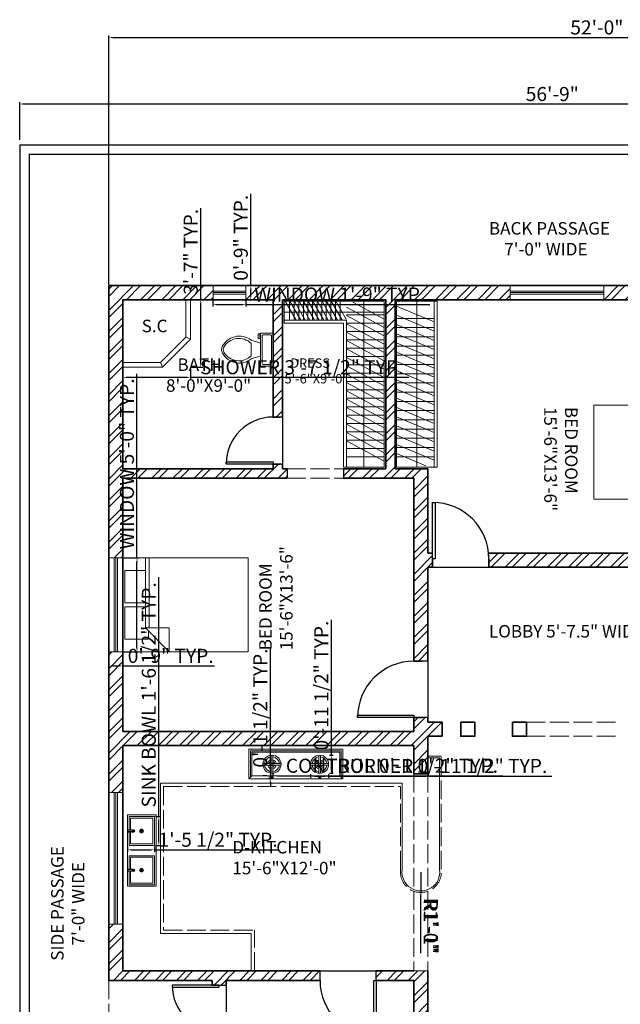
# Model space of a CAD drawing. Units: inches. Extents: x 839 to 1638, y 2998 to 4342.
# Tile 3 of 4: x 839 to 1223, y 3713 to 4342. Entities that reach past the tile are written whole.
import ezdxf

# ---------------------------------------------------------------- set-up
doc = ezdxf.new("R2010")
doc.units = ezdxf.units.IN
doc.linetypes.add('ACAD_ISO02W100', pattern=[15, 12, -3])
for name, color, linetype, lineweight in [('A-ANNO-DIMS', 2, 'Continuous', 18), ('A-AREA-IDEN', 7, 'Continuous', 18), ('A-COLS', 7, 'Continuous', 35), ('A-DOOR', 4, 'Continuous', 25), ('A-DOOR-JAMB', 7, 'Continuous', 25), ('A-EQPM', 8, 'Continuous', 18), ('A-FLOR-CASE', 9, 'Continuous', 20), ('A-FLOR-CASE-HIDN', 9, 'ACAD_ISO02W100', 13), ('A-FLOR-CASE-PATT', 252, 'Continuous', 13), ('A-FLOR-FIXT', 9, 'Continuous', 18), ('A-FLOR-OVHD', 8, 'ACAD_ISO02W100', 18), ('A-FURN', 8, 'Continuous', 18), ('A-WALL', 7, 'Continuous', 35), ('A-WALL-OVHD', 8, 'ACAD_ISO02W100', 18), ('A-WALL-PATT', 252, 'Continuous', 13), ('C-PROP', 7, 'Continuous', 30)]:
    doc.layers.add(name, color=color, linetype=linetype, lineweight=lineweight)
doc.layers.add('A-GLAZ', color=244, linetype='Continuous', lineweight=20, true_color=0x991b1e)
doc.styles.get("Standard").update_dxf_attribs({"font": 'arial.ttf'})
doc.dimstyles.new('ISO-25', dxfattribs={"dimtxt": 9, "dimasz": 2.5, "dimexe": 1.25, "dimexo": 0.625, "dimtad": 1, "dimlunit": 3, "dimtxsty": 'Standard', "dimcen": 2.5, "dimadec": 0, "dimazin": 0, "dimtfac": 1, "dimtmove": 0, "dimatfit": 3, "dimfxl": 1, "dimarcsym": 0})

# ---------------------------------------------------------------- blocks, each defined once
blk = doc.blocks.new('*U2')
for p, q in [((0, 0), (0, -6)), ((40, 0), (40, -6))]:
    blk.add_line(p, q)
blk.add_lwpolyline([(0, 0), (0, 40), (1.75, 40), (1.75, 0)], close=True)
blk.add_arc((0, 0), 40, 0, 90)
blk = doc.blocks.new('*U5')
for p, q in [((0, 0), (0, -6)), ((40, 0), (40, -6))]:
    blk.add_line(p, q)
blk.add_lwpolyline([(0, 0), (0, 40), (1.75, 40), (1.75, 0)], close=True)
blk.add_arc((0, 0), 40, 0, 90)
blk = doc.blocks.new('*U7')
for p, q in [((-40, 0), (-40, 6)), ((0, 0), (0, 6))]:
    blk.add_line(p, q)
blk.add_lwpolyline([(0, 0), (0, -40), (-1.75, -40), (-1.75, 0)], close=True)
blk.add_arc((0, 0), 40, 180, 270)
blk = doc.blocks.new('*U9')
for p, q in [((-40, 0), (-40, 6)), ((0, 0), (0, 6))]:
    blk.add_line(p, q)
blk.add_lwpolyline([(0, 0), (0, -40), (-1.75, -40), (-1.75, 0)], close=True)
blk.add_arc((0, 0), 40, 180, 270)
blk = doc.blocks.new('*U10')
for p, q in [((0, 0), (0, 6)), ((40, 0), (40, 6))]:
    blk.add_line(p, q)
blk.add_lwpolyline([(0, 0), (0, -40), (1.75, -40), (1.75, 0)], close=True)
blk.add_arc((0, 0), 40, 270, 360)
blk = doc.blocks.new('Bed - Queen')
for p, q in [((0, -80.00003), (0, 0)), ((0, 0), (59.99999, 0)), ((59.99999, 0), (59.99999, -80.00003)), ((7.99999, -1.2), (28.79998, -1.2)), ((7.99999, -14.4), (7.99999, -1.2)), ((28.79998, -1.2), (28.79998, -14.4)), ((31.19999, -1.2), (51.99999, -1.2)), ((31.19999, -14.4), (31.19999, -1.2)), ((51.99999, -1.2), (51.99999, -16.4)), ((0, -14.4), (44.8, -14.4)), ((44.8, -16.8), (0, -16.8)), ((59.99999, -29.6), (44.8, -14.4)), ((44.8, -14.4), (44.8, -29.6)), ((51.99999, -16.4), (46.79936, -16.4)), ((44.8, -29.6), (59.99999, -29.6)), ((59.99999, -80.00003), (0, -80.00003))]:
    blk.add_line(p, q)
blk = doc.blocks.new('*U15')
for p, q in [((9.5, -6), (9.5, -2)), ((-10, -8.5), (-8, -8.5)), ((-10, -9.5), (-10, -8.5)), ((-7, -9.5), (-10, -9.5)), ((-8, -8.5), (-8, -8)), ((-7, -8), (-7, -9.5)), ((-4, -8), (-6, -14)), ((4, -8), (6, -14)), ((4, -14), (-4, -14))]:
    blk.add_line(p, q)
blk.add_lwpolyline([(10.5, -8), (10.5, 0), (-10.5, 0), (-10.5, -8)], close=True)
for points in [[(-9.5, -2), (-9.5, -6)], [(8.5, -1), (-8.5, -1)], [(-8.5, -7), (8.5, -7)]]:
    blk.add_lwpolyline(points)
for centre, radius, start, end in [((-8.62, -1.88), 0.884, 81.8699, 188.1301), ((-8.62, -6.12), 0.884, 171.8699, 278.1301), ((8.62, -1.88), 0.884, 351.8699, 98.1301), ((8.62, -6.12), 0.884, 261.8699, 8.1301), ((3.52, -21.58), 12.17, 141.46911, 247.97143), ((4.2, -21.82), 11.33, 136.36773, 238.94682), ((-3.52, -21.58), 12.17, 292.02843, 38.53071), ((-4.2, -21.82), 11.33, 301.05301, 43.63209), ((0, -27.88), 4, 245.73182, 294.26817), ((0, -29), 4, 254.86053, 285.13947)]:
    blk.add_arc(centre, radius, start, end)
blk = doc.blocks.new('*D20')
at = {"layer": 'A-ANNO-DIMS', "color": 0, "lineweight": -2, "transparency": 16777216}
for p, q in [((839.17, 4265.09), (839.17, 4289.16)), ((841.67, 4287.91), (1517.67, 4287.91)), ((1520.17, 4265.46), (1520.17, 4289.16))]:
    blk.add_line(p, q, dxfattribs=at)
at = {"layer": 'A-ANNO-DIMS', "color": 0, "transparency": 16777216}
for points in [[(841.67, 4288.33), (841.67, 4287.5), (839.17, 4287.91)], [(1517.67, 4288.33), (1517.67, 4287.5), (1520.17, 4287.91)]]:
    blk.add_solid(points, dxfattribs=at)
at = {"layer": 'Defpoints', "color": 0, "transparency": 16777216}
for p in [(1520.17, 4287.91), (839.17, 4264.46), (1520.17, 4264.84)]:
    blk.add_point(p, dxfattribs=at)
at = {"layer": 'A-ANNO-DIMS', "color": 0, "transparency": 16777216, "insert": (1179.67, 4293.13), "char_height": 9, "attachment_point": 5}
blk.add_mtext('56\'-9"', dxfattribs=at)
blk = doc.blocks.new('WIN-60x9')
for p, q in [((3.5, 60), (3.5, 0)), ((4.5, 60), (4.5, 0)), ((5.5, 60), (5.5, 0))]:
    blk.add_line(p, q)
blk.add_lwpolyline([(9, 60), (9, 0), (0, 0), (0, 60)], close=True)
blk = doc.blocks.new('WIN-21x9')
for p, q in [((0, 5.5), (21, 5.5)), ((0, 4.5), (21, 4.5)), ((0, 3.5), (21, 3.5))]:
    blk.add_line(p, q)
blk.add_lwpolyline([(0, 9), (21, 9), (21, 0), (0, 0)], close=True)
blk = doc.blocks.new('POST-9x9')
blk.add_lwpolyline([(0, 9), (9, 9), (9, 0), (0, 0)], close=True)
blk = doc.blocks.new('SHOWER-CORNER')
for p, q in [((40.25, 43.12), (40.25, 19.12)), ((43.25, 43.12), (43.25, 17.87)), ((24, 3), (40.25, 19.12)), ((40.25, 19.12), (43.25, 17.87)), ((25.23, 0), (43.25, 17.87)), ((0, 3), (24, 3)), ((0, 0), (25.23, 0)), ((24, 3), (25.23, 0))]:
    blk.add_line(p, q)
blk = doc.blocks.new('SINK-BOWL-WITH-TAP')
for p, q in [((0, 9.97), (3.7, 9.97)), ((0, 9.67), (3.31, 9.67)), ((0, 8.87), (3.31, 8.87)), ((0, 8.57), (3.7, 8.57)), ((7.73, 9.27), (10.16, 9.27)), ((9.8, 8.4), (8.09, 10.14)), ((8.15, 8.35), (9.75, 10.19)), ((8.95, 10.49), (8.95, 8.05))]:
    blk.add_line(p, q)
for points in [[(1, 9.97), (1, 18.54), (17.27, 18.54), (17.27, 0), (1, 0), (1, 8.57)], [(2, 9.97), (2, 17.54), (16.27, 17.54), (16.27, 1), (2, 1), (2, 8.57)]]:
    blk.add_lwpolyline(points)
for centre, radius in [((3.93, 9.27), 0.739), ((3.93, 9.27), 0.439), ((8.95, 9.27), 1.22), ((8.95, 9.27), 0.619)]:
    blk.add_circle(centre, radius)
blk = doc.blocks.new('COOKTOP-BURNER')
for p, q in [((5.27, 11.54), (5.27, 0)), ((6.27, 11.54), (6.27, 0)), ((0, 6.27), (11.54, 6.27)), ((0, 5.27), (11.54, 5.27))]:
    blk.add_line(p, q)
blk.add_circle((5.77, 5.77), 5.77)
for radius, start, end in [(4.77, 96.01576, 173.98424), (2.77, 100.39579, 169.60421), (1.77, 106.40006, 163.59994), (4.77, 6.01576, 83.98424), (2.77, 10.39579, 79.60421), (1.77, 16.40006, 73.59994), (4.77, 186.01576, 263.98424), (2.77, 190.39579, 259.60421), (1.77, 196.40006, 253.59994), (1.77, 286.40006, 343.59994), (2.77, 280.39579, 349.60421), (4.77, 276.01576, 353.98424)]:
    blk.add_arc((5.77, 5.77), radius, start, end)
blk = doc.blocks.new('COOKTOP-CONTROL')
for p, q in [((0.03, 0.97), (1.52, 0.97)), ((0.03, 0.57), (1.52, 0.57))]:
    blk.add_line(p, q)
blk.add_circle((0.77, 0.77), 0.771)
for start, end in [(25.1412, 154.8588), (205.1412, 334.8588)]:
    blk.add_arc((0.77, 0.77), 0.471, start, end)
blk = doc.blocks.new('*D32')
at = {"layer": 'A-ANNO-DIMS', "color": 0, "lineweight": -2, "transparency": 16777216}
for p, q in [((962.76, 4162.21), (962.76, 4158.44)), ((965.26, 4159.69), (981.26, 4159.69)), ((983.76, 4162.21), (983.76, 4158.44)), ((983.76, 4159.69), (1101.4, 4159.69))]:
    blk.add_line(p, q, dxfattribs=at)
at = {"layer": 'A-ANNO-DIMS', "color": 0, "transparency": 16777216}
for points in [[(965.26, 4160.1), (965.26, 4159.27), (962.76, 4159.69)], [(981.26, 4160.1), (981.26, 4159.27), (983.76, 4159.69)]]:
    blk.add_solid(points, dxfattribs=at)
at = {"layer": 'Defpoints', "color": 0, "transparency": 16777216}
for p in [(962.76, 4162.84), (983.76, 4162.84), (983.76, 4159.69)]:
    blk.add_point(p, dxfattribs=at)
at = {"layer": 'A-ANNO-DIMS', "color": 0, "transparency": 16777216, "insert": (1043.83, 4164.97), "char_height": 9, "attachment_point": 5}
blk.add_mtext('WINDOW 1\'-9" TYP.', dxfattribs=at)
blk = doc.blocks.new('*D33')
at = {"layer": 'A-ANNO-DIMS', "color": 0, "lineweight": -2, "transparency": 16777216}
for p, q in [((986.91, 4171.84), (986.91, 4230.45)), ((984.39, 4171.84), (988.16, 4171.84)), ((986.91, 4165.34), (986.91, 4169.34)), ((984.39, 4162.84), (988.16, 4162.84))]:
    blk.add_line(p, q, dxfattribs=at)
at = {"layer": 'A-ANNO-DIMS', "color": 0, "transparency": 16777216}
for points in [[(986.5, 4169.34), (987.33, 4169.34), (986.91, 4171.84)], [(986.5, 4165.34), (987.33, 4165.34), (986.91, 4162.84)]]:
    blk.add_solid(points, dxfattribs=at)
at = {"layer": 'Defpoints', "color": 0, "transparency": 16777216}
for p in [(983.76, 4171.84), (986.91, 4171.84), (983.76, 4162.84)]:
    blk.add_point(p, dxfattribs=at)
at = {"layer": 'A-ANNO-DIMS', "color": 0, "transparency": 16777216, "insert": (981.69, 4202.39), "char_height": 9, "attachment_point": 5, "rotation": 90}
blk.add_mtext('0\'-9" TYP.', dxfattribs=at)
blk = doc.blocks.new('*D36')
at = {"layer": 'A-ANNO-DIMS', "color": 0, "lineweight": -2, "transparency": 16777216}
for p, q in [((914.17, 3997.84), (914.17, 4115.47)), ((905.79, 3997.84), (915.42, 3997.84)), ((914.17, 3940.34), (914.17, 3995.34)), ((905.79, 3937.84), (915.42, 3937.84))]:
    blk.add_line(p, q, dxfattribs=at)
at = {"layer": 'A-ANNO-DIMS', "color": 0, "transparency": 16777216}
for points in [[(913.75, 3995.34), (914.59, 3995.34), (914.17, 3997.84)], [(913.75, 3940.34), (914.59, 3940.34), (914.17, 3937.84)]]:
    blk.add_solid(points, dxfattribs=at)
at = {"layer": 'Defpoints', "color": 0, "transparency": 16777216}
for p in [(905.17, 3997.84), (914.17, 3997.84), (905.17, 3937.84)]:
    blk.add_point(p, dxfattribs=at)
at = {"layer": 'A-ANNO-DIMS', "color": 0, "transparency": 16777216, "insert": (908.89, 4057.9), "char_height": 9, "attachment_point": 5, "rotation": 90}
blk.add_mtext('WINDOW 5\'-0" TYP.', dxfattribs=at)
blk = doc.blocks.new('*D37')
at = {"layer": 'A-ANNO-DIMS', "color": 0, "lineweight": -2, "transparency": 16777216}
for p, q in [((896.17, 3937.21), (896.17, 3927.59)), ((905.17, 3937.21), (905.17, 3927.59)), ((898.67, 3928.84), (902.67, 3928.84)), ((905.17, 3928.84), (963.78, 3928.84))]:
    blk.add_line(p, q, dxfattribs=at)
at = {"layer": 'A-ANNO-DIMS', "color": 0, "transparency": 16777216}
for points in [[(898.67, 3929.25), (898.67, 3928.42), (896.17, 3928.84)], [(902.67, 3929.25), (902.67, 3928.42), (905.17, 3928.84)]]:
    blk.add_solid(points, dxfattribs=at)
at = {"layer": 'Defpoints', "color": 0, "transparency": 16777216}
for p in [(896.17, 3937.84), (905.17, 3937.84), (905.17, 3928.84)]:
    blk.add_point(p, dxfattribs=at)
at = {"layer": 'A-ANNO-DIMS', "color": 0, "transparency": 16777216, "insert": (935.72, 3934.06), "char_height": 9, "attachment_point": 5}
blk.add_mtext('0\'-9" TYP.', dxfattribs=at)
blk = doc.blocks.new('*D38')
at = {"layer": 'A-ANNO-DIMS', "color": 0, "lineweight": -2, "transparency": 16777216}
for p, q in [((905.17, 4119.09), (905.17, 4111.98)), ((948.42, 4119.09), (948.42, 4111.98)), ((907.67, 4113.23), (945.92, 4113.23)), ((948.42, 4113.23), (1088.03, 4113.23))]:
    blk.add_line(p, q, dxfattribs=at)
at = {"layer": 'A-ANNO-DIMS', "color": 0, "transparency": 16777216}
for points in [[(907.67, 4113.65), (907.67, 4112.81), (905.17, 4113.23)], [(945.92, 4113.65), (945.92, 4112.81), (948.42, 4113.23)]]:
    blk.add_solid(points, dxfattribs=at)
at = {"layer": 'Defpoints', "color": 0, "transparency": 16777216}
for p in [(905.17, 4119.72), (948.42, 4119.72), (948.42, 4113.23)]:
    blk.add_point(p, dxfattribs=at)
at = {"layer": 'A-ANNO-DIMS', "color": 0, "transparency": 16777216, "insert": (1019.48, 4118.51), "char_height": 9, "attachment_point": 5}
blk.add_mtext('SHOWER 3\'-7 1/2" TYP.', dxfattribs=at)
blk = doc.blocks.new('*D39')
at = {"layer": 'A-ANNO-DIMS', "color": 0, "lineweight": -2, "transparency": 16777216}
for p, q in [((954.91, 4162.84), (954.91, 4221.44)), ((949.05, 4162.84), (956.16, 4162.84)), ((954.91, 4122.22), (954.91, 4160.34)), ((949.05, 4119.72), (956.16, 4119.72))]:
    blk.add_line(p, q, dxfattribs=at)
at = {"layer": 'A-ANNO-DIMS', "color": 0, "transparency": 16777216}
for points in [[(954.49, 4160.34), (955.33, 4160.34), (954.91, 4162.84)], [(954.49, 4122.22), (955.33, 4122.22), (954.91, 4119.72)]]:
    blk.add_solid(points, dxfattribs=at)
at = {"layer": 'Defpoints', "color": 0, "transparency": 16777216}
for p in [(948.42, 4162.84), (954.91, 4162.84), (948.42, 4119.72)]:
    blk.add_point(p, dxfattribs=at)
at = {"layer": 'A-ANNO-DIMS', "color": 0, "transparency": 16777216, "insert": (949.69, 4193.39), "char_height": 9, "attachment_point": 5, "rotation": 90}
blk.add_mtext('3\'-7" TYP.', dxfattribs=at)
blk = doc.blocks.new('*D40')
at = {"layer": 'A-ANNO-DIMS', "color": 0, "lineweight": -2, "transparency": 16777216}
for p, q in [((928.15, 3832.6), (928.15, 3985.49)), ((926, 3832.6), (929.4, 3832.6)), ((928.15, 3816.56), (928.15, 3830.1)), ((926, 3814.06), (929.4, 3814.06))]:
    blk.add_line(p, q, dxfattribs=at)
at = {"layer": 'A-ANNO-DIMS', "color": 0, "transparency": 16777216}
for points in [[(927.74, 3830.1), (928.57, 3830.1), (928.15, 3832.6)], [(927.74, 3816.56), (928.57, 3816.56), (928.15, 3814.06)]]:
    blk.add_solid(points, dxfattribs=at)
at = {"layer": 'Defpoints', "color": 0, "transparency": 16777216}
for p in [(925.37, 3832.6), (928.15, 3832.6), (925.37, 3814.06)]:
    blk.add_point(p, dxfattribs=at)
at = {"layer": 'A-ANNO-DIMS', "color": 0, "transparency": 16777216, "insert": (922.87, 3910.3), "char_height": 9, "attachment_point": 5, "rotation": 90}
blk.add_mtext('SINK BOWL 1\'-6 1/2" TYP.', dxfattribs=at)
blk = doc.blocks.new('*D41')
at = {"layer": 'A-ANNO-DIMS', "color": 0, "lineweight": -2, "transparency": 16777216}
for p, q in [((908.11, 3813.43), (908.11, 3810.03)), ((925.37, 3813.43), (925.37, 3810.03)), ((910.61, 3811.28), (922.87, 3811.28)), ((925.37, 3811.28), (1004.11, 3811.28))]:
    blk.add_line(p, q, dxfattribs=at)
at = {"layer": 'A-ANNO-DIMS', "color": 0, "transparency": 16777216}
for points in [[(910.61, 3811.69), (910.61, 3810.86), (908.11, 3811.28)], [(922.87, 3811.69), (922.87, 3810.86), (925.37, 3811.28)]]:
    blk.add_solid(points, dxfattribs=at)
at = {"layer": 'Defpoints', "color": 0, "transparency": 16777216}
for p in [(908.11, 3814.06), (925.37, 3814.06), (925.37, 3811.28)]:
    blk.add_point(p, dxfattribs=at)
at = {"layer": 'A-ANNO-DIMS', "color": 0, "transparency": 16777216, "insert": (965.99, 3816.56), "char_height": 9, "attachment_point": 5}
blk.add_mtext('1\'-5 1/2" TYP.', dxfattribs=at)
blk = doc.blocks.new('*D42')
at = {"layer": 'A-ANNO-DIMS', "color": 0, "lineweight": -2, "transparency": 16777216}
for p, q in [((1025.15, 3859.53), (1025.15, 3857.18)), ((1027.65, 3858.43), (1034.19, 3858.43)), ((1036.69, 3859.53), (1036.69, 3857.18)), ((1036.69, 3858.43), (1179.45, 3858.43))]:
    blk.add_line(p, q, dxfattribs=at)
at = {"layer": 'A-ANNO-DIMS', "color": 0, "transparency": 16777216}
for points in [[(1027.65, 3858.84), (1027.65, 3858.01), (1025.15, 3858.43)], [(1034.19, 3858.84), (1034.19, 3858.01), (1036.69, 3858.43)]]:
    blk.add_solid(points, dxfattribs=at)
at = {"layer": 'Defpoints', "color": 0, "transparency": 16777216}
for p in [(1025.15, 3860.16), (1036.69, 3860.16), (1036.69, 3858.43)]:
    blk.add_point(p, dxfattribs=at)
at = {"layer": 'A-ANNO-DIMS', "color": 0, "transparency": 16777216, "insert": (1109.32, 3863.7), "char_height": 9, "attachment_point": 5}
blk.add_mtext('BURNER 0\'-11 1/2" TYP.', dxfattribs=at)
blk = doc.blocks.new('*D43')
at = {"layer": 'A-ANNO-DIMS', "color": 0, "lineweight": -2, "transparency": 16777216}
for p, q in [((1038.42, 3871.7), (1038.42, 3958.27)), ((1037.32, 3871.7), (1039.67, 3871.7)), ((1038.42, 3862.66), (1038.42, 3869.2)), ((1037.32, 3860.16), (1039.67, 3860.16))]:
    blk.add_line(p, q, dxfattribs=at)
at = {"layer": 'A-ANNO-DIMS', "color": 0, "transparency": 16777216}
for points in [[(1038.01, 3869.2), (1038.84, 3869.2), (1038.42, 3871.7)], [(1038.01, 3862.66), (1038.84, 3862.66), (1038.42, 3860.16)]]:
    blk.add_solid(points, dxfattribs=at)
at = {"layer": 'Defpoints', "color": 0, "transparency": 16777216}
for p in [(1036.69, 3871.7), (1038.42, 3871.7), (1036.69, 3860.16)]:
    blk.add_point(p, dxfattribs=at)
at = {"layer": 'A-ANNO-DIMS', "color": 0, "transparency": 16777216, "insert": (1033.14, 3916.24), "char_height": 9, "attachment_point": 5, "rotation": 90}
blk.add_mtext('0\'-11 1/2" TYP.', dxfattribs=at)
blk = doc.blocks.new('*D44')
at = {"layer": 'A-ANNO-DIMS', "color": 0, "lineweight": -2, "transparency": 16777216}
for p, q in [((997.15, 3858.56), (994.65, 3858.56)), ((999.65, 3858.96), (999.65, 3859.81)), ((999.65, 3858.56), (1001.19, 3858.56)), ((1001.19, 3858.96), (1001.19, 3859.81)), ((1003.69, 3858.56), (1148.13, 3858.56))]:
    blk.add_line(p, q, dxfattribs=at)
at = {"layer": 'A-ANNO-DIMS', "color": 0, "transparency": 16777216}
for points in [[(997.15, 3858.98), (997.15, 3858.15), (999.65, 3858.56)], [(1003.69, 3858.98), (1003.69, 3858.15), (1001.19, 3858.56)]]:
    blk.add_solid(points, dxfattribs=at)
at = {"layer": 'Defpoints', "color": 0, "transparency": 16777216}
for p in [(999.65, 3858.33), (1001.19, 3858.56), (1001.19, 3858.33)]:
    blk.add_point(p, dxfattribs=at)
at = {"layer": 'A-ANNO-DIMS', "color": 0, "transparency": 16777216, "insert": (1077.16, 3863.84), "char_height": 9, "attachment_point": 5}
blk.add_mtext('CONTROL 0\'-1 1/2" TYP.', dxfattribs=at)
blk = doc.blocks.new('*D45')
at = {"layer": 'A-ANNO-DIMS', "color": 0, "lineweight": -2, "transparency": 16777216}
for p, q in [((999.42, 3860.83), (999.42, 3940.41)), ((999.02, 3858.33), (998.17, 3858.33)), ((999.42, 3856.79), (999.42, 3858.33)), ((999.02, 3856.79), (998.17, 3856.79)), ((999.42, 3854.29), (999.42, 3851.79))]:
    blk.add_line(p, q, dxfattribs=at)
at = {"layer": 'A-ANNO-DIMS', "color": 0, "transparency": 16777216}
for points in [[(999, 3860.83), (999.83, 3860.83), (999.42, 3858.33)], [(999, 3854.29), (999.83, 3854.29), (999.42, 3856.79)]]:
    blk.add_solid(points, dxfattribs=at)
at = {"layer": 'Defpoints', "color": 0, "transparency": 16777216}
for p in [(999.42, 3858.33), (999.65, 3858.33), (999.65, 3856.79)]:
    blk.add_point(p, dxfattribs=at)
at = {"layer": 'A-ANNO-DIMS', "color": 0, "transparency": 16777216, "insert": (994.14, 3901.87), "char_height": 9, "attachment_point": 5, "rotation": 90}
blk.add_mtext('0\'-1 1/2" TYP.', dxfattribs=at)
blk = doc.blocks.new('*D50')
at = {"layer": 'A-ANNO-DIMS', "color": 0, "lineweight": -2, "transparency": 16777216}
for p, q in [((896.17, 4172.46), (896.17, 4331.69)), ((898.67, 4330.44), (1517.67, 4330.44)), ((1520.17, 4265.46), (1520.17, 4331.69))]:
    blk.add_line(p, q, dxfattribs=at)
at = {"layer": 'A-ANNO-DIMS', "color": 0, "transparency": 16777216}
for points in [[(898.67, 4330.85), (898.67, 4330.02), (896.17, 4330.44)], [(1517.67, 4330.85), (1517.67, 4330.02), (1520.17, 4330.44)]]:
    blk.add_solid(points, dxfattribs=at)
at = {"layer": 'Defpoints', "color": 0, "transparency": 16777216}
for p in [(1520.17, 4330.44), (1520.17, 4264.84), (896.17, 4171.84)]:
    blk.add_point(p, dxfattribs=at)
at = {"layer": 'A-ANNO-DIMS', "color": 0, "transparency": 16777216, "insert": (1208.17, 4335.66), "char_height": 9, "attachment_point": 5}
blk.add_mtext('52\'-0"', dxfattribs=at)
blk = doc.blocks.new('*D52')
at = {"layer": 'A-ANNO-DIMS', "color": 0, "lineweight": -2, "transparency": 16777216}
for p, q in [((1095.67, 3797.09), (1095.67, 3783.99)), ((1095.67, 3745.2), (1095.67, 3781.49))]:
    blk.add_line(p, q, dxfattribs=at)
at = {"layer": 'A-ANNO-DIMS', "color": 0, "transparency": 16777216}
blk.add_solid([(1096.09, 3781.49), (1095.25, 3781.49), (1095.67, 3783.99)], dxfattribs=at)
at = {"layer": 'Defpoints', "color": 0, "transparency": 16777216}
for p in [(1095.67, 3797.09), (1095.67, 3783.99)]:
    blk.add_point(p, dxfattribs=at)
at = {"layer": 'A-ANNO-DIMS', "color": 0, "transparency": 16777216, "insert": (1100.81, 3762.1), "char_height": 9, "attachment_point": 5, "rotation": 270.00202}
blk.add_mtext('R1\'-1"', dxfattribs=at)
blk = doc.blocks.new('*D53')
at = {"layer": 'A-ANNO-DIMS', "color": 0, "lineweight": -2, "transparency": 16777216}
for p, q in [((1095.67, 3797.09), (1095.67, 3784.99)), ((1095.67, 3746.2), (1095.67, 3782.49))]:
    blk.add_line(p, q, dxfattribs=at)
at = {"layer": 'A-ANNO-DIMS', "color": 0, "transparency": 16777216}
blk.add_solid([(1096.09, 3782.49), (1095.25, 3782.49), (1095.67, 3784.99)], dxfattribs=at)
at = {"layer": 'Defpoints', "color": 0, "transparency": 16777216}
for p in [(1095.67, 3797.09), (1095.67, 3784.99)]:
    blk.add_point(p, dxfattribs=at)
at = {"layer": 'A-ANNO-DIMS', "color": 0, "transparency": 16777216, "insert": (1100.89, 3763.1), "char_height": 9, "attachment_point": 5, "rotation": 270.00219}
blk.add_mtext('R1\'-0"', dxfattribs=at)

msp = doc.modelspace()

# ---------------------------------------------------------------- hatches: boundary and pattern name
at = {"layer": 'A-FLOR-CASE-PATT'}
h = msp.add_hatch(dxfattribs=at)
h.set_pattern_fill('ANSI31', color=256, scale=0.8000071, angle=74.98736, style=0)
h.paths.add_polyline_path([(1008.169, 4161.836), (1015.093, 4149.836), (1047.352, 4149.836), (1049.079, 4151.925), (1043.36, 4161.836)])
h = msp.add_hatch(dxfattribs=at)
h.set_pattern_fill('ANSI31', color=256, scale=0.923651, angle=45, style=0)
h.paths.add_polyline_path([(1011.101, 4149.836), (1046.292, 4149.836), (1046.292, 4161.836), (1011.101, 4161.836)])
h = msp.add_hatch(dxfattribs=at)
h.set_pattern_fill('ANSI31', color=256, scale=1.4792288, angle=106.61663, style=0)
h.paths.add_polyline_path([(1072.169, 4055.836), (1072.169, 4151.925), (1053.826, 4161.836), (1048.169, 4159.554), (1048.169, 4068.804)])
h = msp.add_hatch(dxfattribs=at)
h.set_pattern_fill('ANSI31', color=256, scale=1.709775, angle=112.0271, style=0)
h.paths.add_polyline_path([(1104.169, 4151.662), (1080.169, 4161.836), (1080.169, 4061.666), (1093.923, 4055.836), (1104.169, 4057.389)])
h = msp.add_hatch(dxfattribs=at)
h.set_pattern_fill('ANSI31', color=256, scale=1.68135, angle=-45, style=0)
h.paths.add_polyline_path([(1072.169, 4061.174), (1072.169, 4157.263), (1048.169, 4157.263), (1048.169, 4061.174)])
h = msp.add_hatch(dxfattribs=at)
h.set_pattern_fill('ANSI31', color=256, scale=1.85706, angle=-45, style=0)
h.paths.add_polyline_path([(1104.169, 4155.94), (1080.169, 4155.94), (1080.169, 4061.666), (1104.169, 4061.666)])
at = {"layer": 'A-WALL-PATT'}
h = msp.add_hatch(dxfattribs=at)
h.set_pattern_fill('ANSI32', color=256)
h.paths.add_polyline_path([(1440.674, 3673.836), (1430.169, 3673.836), (1430.169, 3724.836), (1421.169, 3724.836), (1421.169, 3673.836), (1209.669, 3673.836), (1209.669, 3670.236), (1209.669, 3664.836), (1247.169, 3664.836), (1247.169, 3661.836), (1252.569, 3661.836), (1256.169, 3661.836), (1256.169, 3664.836), (1440.674, 3664.836)])
h.paths.add_polyline_path([(1137.669, 3673.836), (1100.169, 3673.836), (1100.169, 3733.836), (1091.169, 3733.836), (1067.169, 3733.836), (1067.169, 3727.836), (1091.169, 3727.836), (1091.169, 3640.836), (971.169, 3640.836), (971.169, 3694.836), (962.169, 3694.836), (962.169, 3640.836), (896.169, 3640.836), (896.169, 3628.836), (905.169, 3628.836), (905.169, 3631.836), (1091.169, 3631.836), (1091.169, 3628.836), (1100.169, 3628.836), (1100.169, 3664.836), (1137.669, 3664.836)])
h.paths.add_polyline_path([(1256.169, 3625.836), (1247.169, 3625.836), (1247.169, 3491.75), (1237.967, 3478.332), (1245.508, 3473.161), (1247.169, 3475.836), (1520.169, 3475.836), (1520.169, 3595.836), (1504.368, 3595.836), (1504.368, 3586.836), (1511.169, 3586.836), (1511.169, 3484.836), (1439.169, 3484.836), (1439.169, 3550.955), (1415.169, 3550.955), (1415.169, 3586.836), (1418.169, 3586.836), (1418.169, 3595.836), (1406.169, 3595.836), (1406.169, 3544.955), (1433.169, 3544.955), (1433.169, 3484.836), (1406.169, 3484.836), (1256.169, 3484.836)])
h.paths.add_polyline_path([(1483.368, 3595.836), (1472.169, 3595.836), (1472.169, 3600.336), (1463.169, 3600.336), (1463.169, 3595.836), (1448.169, 3595.836), (1448.169, 3586.836), (1483.368, 3586.836)], flags=17)
h.paths.add_polyline_path([(1220.169, 3432.336), (1210.822, 3438.745), (1206.427, 3432.336), (1179.669, 3432.336), (1179.669, 3423.336), (1211.169, 3423.336), (1211.169, 3298.836), (1367.169, 3298.836), (1367.169, 3307.836), (1220.169, 3307.836)])
h.paths.add_polyline_path([(1041.669, 3532.086), (1058.169, 3532.086), (1058.169, 3541.086), (1032.669, 3541.086), (1032.669, 3432.336), (905.169, 3432.336), (905.169, 3470.704), (896.169, 3470.704), (896.169, 3423.336), (1055.555, 3423.336), (1055.555, 3432.336), (1041.669, 3432.336)])
h.paths.add_polyline_path([(1100.169, 3592.836), (1091.169, 3592.836), (1091.169, 3541.086), (1088.169, 3541.086), (1088.169, 3532.086), (1091.169, 3532.086), (1091.169, 3432.336), (1076.555, 3432.336), (1076.555, 3423.336), (1100.169, 3423.336), (1107.669, 3423.336), (1107.669, 3432.336), (1100.169, 3432.336)])
h.paths.add_polyline_path([(905.169, 3592.836), (896.169, 3592.836), (896.169, 3566.704), (905.169, 3566.704)])
h.paths.add_polyline_path([(905.169, 3763.836), (896.169, 3763.836), (896.169, 3727.836), (962.169, 3727.836), (962.169, 3724.836), (971.169, 3724.836), (971.169, 3727.836), (1031.169, 3727.836), (1031.169, 3733.836), (905.169, 3733.836)])
h.paths.add_polyline_path([(1109.169, 3892.836), (1100.169, 3892.836), (1100.169, 3895.836), (1091.169, 3895.836), (1091.169, 3886.836), (905.169, 3886.836), (905.169, 3937.836), (896.169, 3937.836), (896.169, 3847.836), (905.169, 3847.836), (905.169, 3877.836), (1091.169, 3877.836), (1091.169, 3859.836), (1100.169, 3859.836), (1100.169, 3883.836), (1109.169, 3883.836)])
h.paths.add_polyline_path([(905.169, 4162.836), (962.764, 4162.836), (962.764, 4171.836), (896.169, 4171.836), (896.169, 3997.836), (905.169, 3997.836), (905.169, 4048.836), (1010.169, 4048.836), (1010.169, 4054.836), (1007.169, 4054.836), (1007.169, 4057.836), (1001.169, 4057.836), (1001.169, 4054.836), (905.169, 4054.836)])
h.paths.add_polyline_path([(1152.669, 4171.836), (983.764, 4171.836), (983.764, 4162.836), (1001.169, 4162.836), (1001.169, 4087.836), (1007.169, 4087.836), (1007.169, 4162.836), (1073.169, 4162.836), (1073.169, 4054.836), (1046.169, 4054.836), (1046.169, 4048.836), (1091.169, 4048.836), (1091.169, 3931.836), (1100.169, 3931.836), (1100.169, 3991.836), (1103.169, 3991.836), (1103.169, 4000.836), (1100.169, 4000.836), (1100.169, 4054.836), (1079.169, 4054.836), (1079.169, 4162.836), (1152.669, 4162.836)])
h.paths.add_polyline_path([(1336.119, 4171.836), (1212.669, 4171.836), (1212.669, 4162.836), (1286.169, 4162.836), (1286.169, 4159.836), (1295.169, 4159.836), (1295.169, 4162.836), (1336.119, 4162.836)], flags=17)
h.paths.add_polyline_path([(1295.169, 4129.836), (1286.169, 4129.836), (1286.169, 4000.836), (1139.169, 4000.836), (1139.169, 3991.836), (1286.169, 3991.836), (1286.169, 3931.836), (1295.169, 3931.836), (1295.169, 4072.836), (1451.169, 4072.836), (1451.169, 4078.836), (1421.169, 4078.836), (1421.169, 4141.836), (1452.669, 4141.836), (1452.669, 4147.836), (1424.169, 4147.836), (1397.169, 4171.836), (1397.169, 4199.532), (1388.169, 4199.532), (1388.169, 4171.836), (1357.119, 4171.836), (1357.119, 4162.836), (1398.069, 4162.836), (1415.169, 4147.29), (1415.169, 4078.836), (1295.169, 4078.836)])
h.paths.add_polyline_path([(1442.169, 3892.836), (1295.169, 3892.836), (1295.169, 3895.836), (1286.169, 3895.836), (1286.169, 3892.836), (1277.169, 3892.836), (1277.169, 3883.836), (1421.169, 3883.836), (1421.169, 3832.836), (1430.169, 3832.836), (1430.169, 3883.836), (1442.169, 3883.836)])
h.paths.add_polyline_path([(1520.169, 4264.836), (1388.169, 4264.836), (1388.169, 4220.532), (1397.169, 4220.532), (1397.169, 4255.836), (1511.169, 4255.836), (1511.169, 4147.836), (1482.669, 4147.836), (1482.669, 4141.836), (1511.169, 4141.836), (1511.169, 4078.836), (1481.169, 4078.836), (1481.169, 4072.836), (1511.169, 4072.836), (1511.169, 3892.836), (1502.169, 3892.836), (1502.169, 3883.836), (1514.169, 3883.836), (1514.169, 3724.836), (1520.169, 3724.836)])
h.paths.add_polyline_path([(1319.528, 4099.601), (1381.705, 4099.601), (1381.705, 4129.453), (1319.528, 4129.453)], flags=25)

# ---------------------------------------------------------------- linework, layer by layer
at = {"layer": 'A-DOOR'}
for p, q in [((1007.169, 4087.836), (1007.169, 4057.836)), ((1103.169, 3991.836), (1139.169, 3991.836)), ((1100.169, 3931.836), (1100.169, 3895.836)), ((1031.169, 3733.836), (1067.169, 3733.836)), ((971.169, 3724.836), (971.169, 3694.836))]:
    msp.add_line(p, q, dxfattribs=at)
at = {"layer": 'A-DOOR-JAMB'}
for p, q in [((1007.169, 4087.836), (1001.169, 4087.836)), ((1007.169, 4057.836), (1001.169, 4057.836)), ((1010.169, 4054.836), (1010.169, 4048.836)), ((1046.169, 4054.836), (1046.169, 4048.836)), ((1103.169, 3991.836), (1103.169, 4000.836)), ((1139.169, 3991.836), (1139.169, 4000.836)), ((1100.169, 3931.836), (1091.169, 3931.836)), ((1100.169, 3895.836), (1091.169, 3895.836)), ((1031.169, 3727.836), (1031.169, 3733.836)), ((1067.169, 3727.836), (1067.169, 3733.836)), ((962.169, 3724.836), (971.169, 3724.836))]:
    msp.add_line(p, q, dxfattribs=at)
at = {"layer": 'A-EQPM'}
for p, q in [((985.652, 3856.652), (987.652, 3858.652)), ((1045.745, 3856.652), (1043.745, 3858.652))]:
    msp.add_line(p, q, dxfattribs=at)
for points in [[(985.652, 3875.627), (1045.745, 3875.627), (1045.745, 3856.652), (985.652, 3856.652)], [(987.652, 3873.627), (1043.745, 3873.627), (1043.745, 3858.652), (987.652, 3858.652)]]:
    msp.add_lwpolyline(points, close=True, dxfattribs=at)
msp.add_lwpolyline([(986.652, 3857.652), (986.652, 3874.627), (1044.745, 3874.627), (1044.745, 3857.652)], dxfattribs=at)
at = {"layer": 'A-FLOR-CASE'}
for p, q in [((1008.169, 4161.836), (1072.169, 4161.836)), ((1008.169, 4161.836), (1008.169, 4147.836)), ((1059.169, 4055.836), (1059.169, 4161.836)), ((1072.169, 4161.836), (1072.169, 4055.836)), ((1080.169, 4161.836), (1080.169, 4055.836)), ((1080.169, 4161.836), (1106.169, 4161.836)), ((1093.169, 4055.836), (1093.169, 4161.836)), ((1104.169, 4161.836), (1104.169, 4055.836)), ((1106.169, 4161.836), (1106.169, 4055.836)), ((1008.169, 4154.836), (1072.169, 4154.836)), ((1008.169, 4149.836), (1048.169, 4149.836)), ((1008.169, 4147.836), (1046.169, 4147.836)), ((1046.169, 4147.836), (1046.169, 4055.836)), ((1048.169, 4149.836), (1048.169, 4055.836)), ((1046.169, 4055.836), (1072.169, 4055.836)), ((1080.169, 4055.836), (1106.169, 4055.836)), ((1107.669, 3870.099), (1100.169, 3870.099)), ((1107.669, 3798.609), (1107.669, 3870.099)), ((1107.669, 3870.099), (1107.669, 3870.099)), ((929.169, 3853.836), (1083.669, 3853.836)), ((929.169, 3853.836), (929.169, 3757.836)), ((1083.669, 3798.609), (1083.669, 3853.836)), ((929.169, 3757.836), (987.2, 3757.836)), ((987.2, 3733.836), (987.2, 3757.836))]:
    msp.add_line(p, q, dxfattribs=at)
msp.add_arc((1095.669, 3797.088), 12.096, 172.775635, 7.224365, dxfattribs=at)
at = {"layer": 'A-FLOR-CASE-HIDN'}
for p, q in [((1108.669, 3871.099), (1100.169, 3871.099)), ((1108.669, 3798.671), (1108.669, 3871.099)), ((931.169, 3851.836), (931.169, 3759.836)), ((931.169, 3851.836), (1082.669, 3851.836)), ((1082.669, 3798.671), (1082.669, 3851.836)), ((931.169, 3759.836), (989.2, 3759.836)), ((989.2, 3733.836), (989.2, 3759.836))]:
    msp.add_line(p, q, dxfattribs=at)
msp.add_arc((1095.669, 3797.088), 13.096, 173.057286, 6.942714, dxfattribs=at)
at = {"layer": 'A-FLOR-FIXT'}
msp.add_lwpolyline([(908.108, 3833.598), (926.374, 3833.598), (926.374, 3787.97), (908.108, 3787.97)], close=True, dxfattribs=at)
at = {"layer": 'A-FLOR-OVHD'}
for p, q in [((1163.169, 3892.836), (1223.169, 3892.836)), ((1163.169, 3883.836), (1223.169, 3883.836)), ((1091.169, 3859.836), (1091.169, 3733.836)), ((1100.169, 3859.836), (1100.169, 3733.836))]:
    msp.add_line(p, q, dxfattribs=at)
at = {"layer": 'A-GLAZ'}
for p, q in [((899.669, 3847.836), (899.669, 3763.836)), ((900.669, 3847.836), (900.669, 3763.836)), ((901.669, 3847.836), (901.669, 3763.836))]:
    msp.add_line(p, q, dxfattribs=at)
msp.add_lwpolyline([(905.169, 3847.836), (905.169, 3763.836), (896.169, 3763.836), (896.169, 3847.836)], close=True, dxfattribs=at)
at = {"layer": 'A-WALL'}
for p, q in [((896.169, 4171.836), (896.169, 3727.836)), ((896.169, 4171.836), (1388.169, 4171.836)), ((905.169, 4162.836), (1001.169, 4162.836)), ((905.169, 4162.836), (905.169, 4054.836)), ((1001.169, 4162.836), (1001.169, 4087.836)), ((1007.169, 4162.836), (1007.169, 4087.836)), ((1007.169, 4162.836), (1073.169, 4162.836)), ((1073.169, 4162.836), (1073.169, 4054.836)), ((1079.169, 4162.836), (1079.169, 4054.836)), ((1079.169, 4162.836), (1286.169, 4162.836)), ((905.169, 4054.836), (1001.169, 4054.836)), ((1001.169, 4057.836), (1001.169, 4054.836)), ((1007.169, 4057.836), (1007.169, 4054.836)), ((1007.169, 4054.836), (1010.169, 4054.836)), ((1046.169, 4054.836), (1073.169, 4054.836)), ((1079.169, 4054.836), (1100.169, 4054.836)), ((1100.169, 4054.836), (1100.169, 4000.836)), ((905.169, 4048.836), (1010.169, 4048.836)), ((905.169, 4048.836), (905.169, 3886.836)), ((1046.169, 4048.836), (1091.169, 4048.836)), ((1091.169, 4048.836), (1091.169, 3931.836)), ((1100.169, 4000.836), (1103.169, 4000.836)), ((1139.169, 4000.836), (1286.169, 4000.836)), ((1100.169, 3991.836), (1103.169, 3991.836)), ((1100.169, 3991.836), (1100.169, 3931.836)), ((1139.169, 3991.836), (1286.169, 3991.836)), ((1091.169, 3895.836), (1091.169, 3886.836)), ((1100.169, 3895.836), (1100.169, 3892.836)), ((1100.169, 3892.836), (1109.169, 3892.836)), ((1109.169, 3892.836), (1109.169, 3883.836)), ((905.169, 3886.836), (1091.169, 3886.836)), ((1100.169, 3883.836), (1100.169, 3859.836)), ((1100.169, 3883.836), (1109.169, 3883.836)), ((905.169, 3877.836), (1091.169, 3877.836)), ((905.169, 3877.836), (905.169, 3733.836)), ((1091.169, 3877.836), (1091.169, 3859.836)), ((1091.169, 3859.836), (1100.169, 3859.836)), ((905.169, 3733.836), (1031.169, 3733.836)), ((1067.169, 3733.836), (1091.169, 3733.836)), ((1100.169, 3733.836), (1100.169, 3673.836)), ((896.169, 3727.836), (962.169, 3727.836)), ((962.169, 3727.836), (962.169, 3724.836)), ((971.169, 3727.836), (971.169, 3724.836)), ((971.169, 3727.836), (1031.169, 3727.836)), ((1067.169, 3727.836), (1091.169, 3727.836)), ((1091.169, 3727.836), (1091.169, 3640.836))]:
    msp.add_line(p, q, dxfattribs=at)
at = {"layer": 'A-WALL-OVHD'}
for p, q in [((1010.169, 4054.836), (1046.169, 4054.836)), ((1010.169, 4048.836), (1046.169, 4048.836)), ((1091.169, 3733.836), (1100.169, 3733.836)), ((896.169, 3727.836), (896.169, 3640.836))]:
    msp.add_line(p, q, dxfattribs=at)
at = {"layer": 'C-PROP'}
for p, q in [((839.169, 4261.836), (839.169, 3061.836)), ((839.169, 4261.836), (1388.169, 4261.836)), ((845.169, 4255.836), (1388.169, 4255.836)), ((845.169, 4255.836), (845.169, 3432.336))]:
    msp.add_line(p, q, dxfattribs=at)

# ---------------------------------------------------------------- block references
at = {"layer": 'A-COLS'}
for p in [(1121.169, 3883.836), (1154.169, 3883.836)]:
    msp.add_blockref('POST-9x9', p, dxfattribs=at)
at = {"layer": 'A-DOOR'}
for name, p, xscale, yscale, zscale, rotation in [('*U9', (1001.169, 4057.836), 0.7499999999999982, 0.7499999999999982, 0.7499999999999982, 270), ('*U5', (1091.169, 3895.836), 0.900000000000001, 0.900000000000001, 0.900000000000001, 90), ('*U10', (966.669, 3724.836), 0.75, 0.75, 0.75, 269.9999999999993)]:
    msp.add_blockref(name, p, dxfattribs=dict(at, xscale=xscale, yscale=yscale, zscale=zscale, rotation=rotation))
at = {"layer": 'A-DOOR', "xscale": 0.9, "yscale": 0.9, "zscale": 0.9}
for name, p in [('*U2', (1103.169, 3997.236)), ('*U7', (1067.169, 3727.836))]:
    msp.add_blockref(name, p, dxfattribs=at)
at = {"layer": 'A-EQPM'}
for name, p in [('COOKTOP-BURNER', (994.706, 3860.157)), ('COOKTOP-BURNER', (1025.15, 3860.157)), ('COOKTOP-CONTROL', (999.647, 3856.789)), ('COOKTOP-CONTROL', (1030.208, 3856.789))]:
    msp.add_blockref(name, p, dxfattribs=at)
at = {"layer": 'A-FLOR-FIXT'}
for name, p in [('SHOWER-CORNER', (905.169, 4119.718)), ('SINK-BOWL-WITH-TAP', (908.108, 3814.059))]:
    msp.add_blockref(name, p, dxfattribs=at)
at = {"layer": 'A-FLOR-FIXT', "rotation": 270}
msp.add_blockref('*U15', (1001.169, 4130.956), dxfattribs=at)
at = {"layer": 'A-FLOR-FIXT', "extrusion": (0, 0, -1), "zscale": -1, "rotation": 180}
msp.add_blockref('SINK-BOWL-WITH-TAP', (-908.108, 3807.509), dxfattribs=at)
at = {"layer": 'A-FURN', "rotation": 270}
msp.add_blockref('Bed - Queen', (1286.169, 4095.336), dxfattribs=at)
at = {"layer": 'A-FURN', "xscale": -1, "rotation": 90}
msp.add_blockref('Bed - Queen', (905.169, 3997.836), dxfattribs=at)
at = {"layer": 'A-GLAZ'}
for name, p in [('WIN-21x9', (962.763, 4162.836)), ('WIN-60x9', (896.169, 3937.836))]:
    msp.add_blockref(name, p, dxfattribs=at)
at = {"layer": 'A-GLAZ', "rotation": 89.99999999999653}
msp.add_blockref('WIN-60x9', (1212.668, 4162.836), dxfattribs=at)

# ---------------------------------------------------------------- texts
at = {"layer": 'A-AREA-IDEN', "attachment_point": 1}
for s, width, insert, char_height in [('BACK PASSAGE\\P    7\'-0" WIDE', 89.64254, (1139.169, 4212.448), 8), ('S.C', 16.07573, (917.169, 4150.057), 8), ('   BATH\\P8\'-0"X9\'-0"', 51.99955, (932.7, 4125.336), 8), ('  DRESS\\P5\'-6"X9\'-0"', 38.08759, (1008.485, 4125.336), 6), ('LOBBY 5\'-7.5" WIDE', 104.90723, (1139.169, 3954.925), 8), ('D-KITCHEN\\P15\'-6"X12\'-0"', 66.18672, (975.173, 3816.937), 8)]:
    msp.add_mtext_dynamic_manual_height_columns(s, width=width, gutter_width=12.5, heights=[0], dxfattribs=dict(at, insert=insert, char_height=char_height))
at = {"layer": 'A-AREA-IDEN', "char_height": 8, "attachment_point": 1}
for s, width, insert, rotation in [('BED ROOM\\P15\'-6"X13\'-6"', 66.18672, (1195.826, 4094.335), 270), ('BED ROOM\\P15\'-6"X13\'-6"', 66.18672, (992.308, 3938.783), 90), ('SIDE PASSAGE\\P    7\'-0" WIDE', 89.64254, (859.241, 3740.394), 90)]:
    msp.add_mtext_dynamic_manual_height_columns(s, width=width, gutter_width=12.5, heights=[0], dxfattribs=dict(at, insert=insert, rotation=rotation))

# ---------------------------------------------------------------- dimensions: what is measured, and where the dimension line sits
at = {"layer": 'A-ANNO-DIMS'}
for base, p1, override, picture, middle in [((1520.169, 4330.436), (896.169, 4171.836), {"dimdec": 1, "dimlfac": 1, "dimrnd": 0, "dimzin": 1, "dimdsep": 46, "dimlunit": 4, "dimfrac": 2}, '*D50', (1208.169, 4335.656)), ((1520.169, 4287.912), (839.169, 4264.461), {"dimclrd": 0, "dimclre": 0, "dimclrt": 0}, '*D20', (1179.669, 4293.132))]:
    dim = msp.add_linear_dim(base=base, p1=p1, p2=(1520.169, 4264.836), dimstyle='ISO-25', override=override, dxfattribs=at)
    dim.commit()
    dim.dimension.update_dxf_attribs({"geometry": picture, "text_midpoint": middle})
for base, p1, p2, text, picture, middle in [((986.914, 4171.836), (983.764, 4162.836), (983.764, 4171.836), '<> TYP.', '*D33', (981.694, 4202.391)), ((954.909, 4162.836), (948.421, 4119.718), (948.421, 4162.836), '<> TYP.', '*D39', (949.685, 4193.387)), ((914.169, 3997.836), (905.169, 3937.836), (905.169, 3997.836), 'WINDOW <> TYP.', '*D36', (908.887, 4057.905)), ((928.155, 3832.598), (925.374, 3814.059), (925.374, 3832.598), 'SINK BOWL <> TYP.', '*D40', (922.873, 3910.296)), ((1038.423, 3871.699), (1036.691, 3860.157), (1036.691, 3871.699), '<> TYP.', '*D43', (1033.144, 3916.236)), ((999.416, 3858.331), (999.647, 3856.789), (999.647, 3858.331), '<> TYP.', '*D45', (994.138, 3901.871))]:
    dim = msp.add_linear_dim(base=base, p1=p1, p2=p2, angle=90, text=text, dimstyle='ISO-25', override={"dimdec": 1, "dimlfac": 1, "dimrnd": 0, "dimzin": 1, "dimdsep": 46, "dimlunit": 4, "dimfrac": 2}, dxfattribs=at)
    dim.commit()
    dim.dimension.update_dxf_attribs({"geometry": picture, "text_midpoint": middle})
for base, p1, p2, text, picture, middle in [((983.764, 4159.686), (962.764, 4162.836), (983.764, 4162.836), 'WINDOW <> TYP.', '*D32', (1043.833, 4164.967)), ((948.421, 4113.23), (905.169, 4119.718), (948.421, 4119.718), 'SHOWER <> TYP.', '*D38', (1019.476, 4118.515)), ((905.169, 3928.836), (896.169, 3937.836), (905.169, 3937.836), '<> TYP.', '*D37', (935.723, 3934.056)), ((1001.189, 3858.562), (999.647, 3858.331), (1001.189, 3858.331), 'CONTROL <> TYP.', '*D44', (1077.159, 3863.844)), ((1036.691, 3858.426), (1025.15, 3860.157), (1036.691, 3860.157), 'BURNER <> TYP.', '*D42', (1109.321, 3863.705)), ((925.374, 3811.278), (908.108, 3814.059), (925.374, 3814.059), '<> TYP.', '*D41', (965.99, 3816.556))]:
    dim = msp.add_linear_dim(base=base, p1=p1, p2=p2, text=text, dimstyle='ISO-25', override={"dimdec": 1, "dimlfac": 1, "dimrnd": 0, "dimzin": 1, "dimdsep": 46, "dimlunit": 4, "dimfrac": 2}, dxfattribs=at)
    dim.commit()
    dim.dimension.update_dxf_attribs({"geometry": picture, "text_midpoint": middle})
for mpoint, picture, middle in [((1095.669, 3783.992), '*D52', (1100.813, 3762.098)), ((1095.669, 3784.992), '*D53', (1100.89, 3763.098))]:
    dim = msp.add_radius_dim(center=(1095.669, 3797.088), mpoint=mpoint, dimstyle='ISO-25', override={"dimdec": 1, "dimlfac": 1, "dimrnd": 0, "dimzin": 1, "dimdsep": 46, "dimlunit": 4, "dimfrac": 2}, dxfattribs=at)
    dim.commit()
    dim.dimension.update_dxf_attribs({"geometry": picture, "text_midpoint": middle})

doc.saveas('drawing.dxf')
